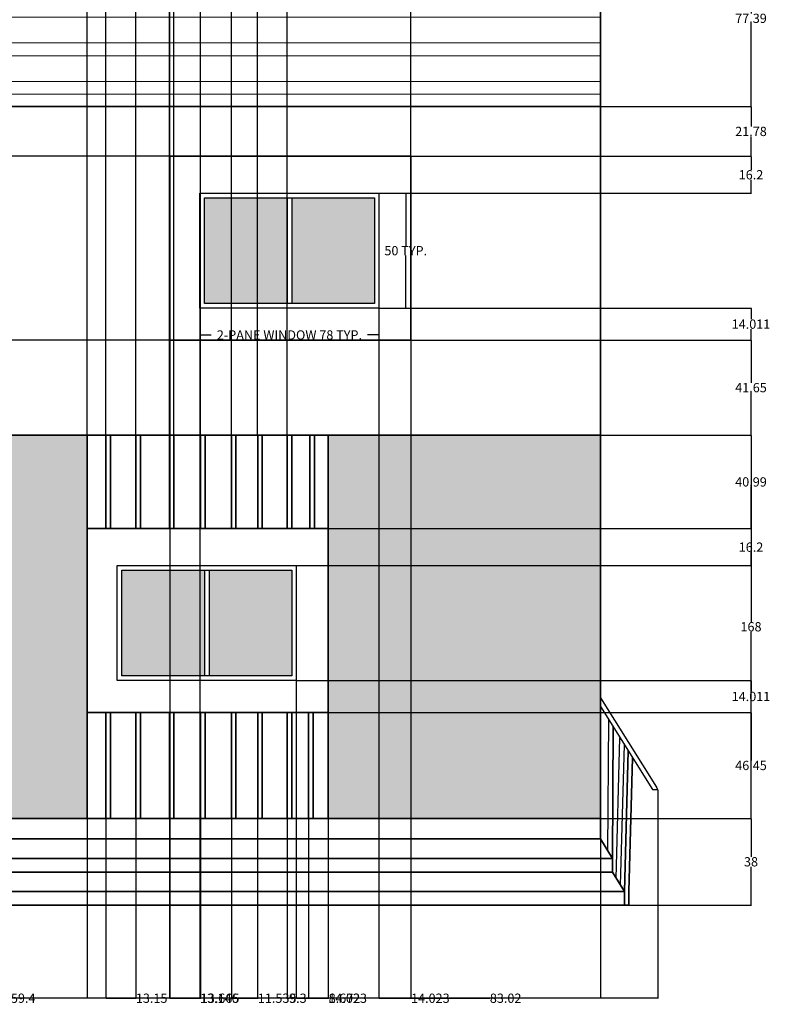
# Model space of a CAD drawing. Units: inches. Extents: x -35 to 623, y 74 to 964.
# Tile 2 of 3: x 294 to 623, y 74 to 505. Entities that reach past the tile are written whole.
import ezdxf

# ---------------------------------------------------------------- set-up
doc = ezdxf.new("R2010")
doc.units = ezdxf.units.IN
doc.header["$MEASUREMENT"] = 0
for name, color, linetype, lineweight in [('A-ANNO-DIMS', 2, 'Continuous', 18), ('A-ELEV', 7, 'Continuous', 35), ('A-ELEV-PATT', 8, 'Continuous', 13), ('A-FLOR-STRS', 7, 'Continuous', 25), ('A-GLAZ', 4, 'Continuous', 25)]:
    doc.layers.add(name, color=color, linetype=linetype, lineweight=lineweight)
doc.styles.get("Standard").update_dxf_attribs({"font": 'arial.ttf'})
doc.dimstyles.get("Standard").update_dxf_attribs({"dimtxt": 4.0625, "dimasz": 0.18, "dimexe": 0.18, "dimexo": 0.0625, "dimgap": 0.09, "dimtad": 0, "dimtih": 1, "dimtoh": 1, "dimdec": 4, "dimzin": 0, "dimdsep": 46, "dimlunit": 4, "dimtxsty": 'Standard', "dimcen": 0.09, "dimadec": 0, "dimazin": 0, "dimtfac": 1, "dimtdec": 4, "dimtofl": 0, "dimtmove": 0, "dimatfit": 3, "dimfxl": 1, "dimtolj": 1, "dimtzin": 0, "dimarcsym": 0})

# ---------------------------------------------------------------- blocks, each defined once
blk = doc.blocks.new('WIN-2PANE')
for p, q in [((38.22, 48.35), (38.22, 2)), ((40.22, 48.35), (40.22, 2))]:
    blk.add_line(p, q)
for points in [[(0, 50.35), (78.44, 50.35), (78.44, 0), (0, 0)], [(2, 48.35), (76.44, 48.35), (76.44, 2), (2, 2)]]:
    blk.add_lwpolyline(points, close=True)
blk = doc.blocks.new('STAIR-RAIL')
for p, q in [((25.22, 82.16), (0.67, 43)), ((25.22, 78.4), (2.36, 41.93)), ((21.93, 15.01), (21.56, 72.56)), ((16.35, 0), (14.7, 61.62)), ((18.27, 3.03), (16.62, 64.68)), ((0, 41.93), (0.67, 43)), ((2.36, 41.93), (0, 41.93))]:
    blk.add_line(p, q)
blk = doc.blocks.new('*D9')
at = {"layer": 'A-ANNO-DIMS', "color": 0, "lineweight": -2, "transparency": 16777216}
for p, q in [((372.93, 378.73), (372.93, 366.84)), ((451.37, 378.73), (451.37, 366.84)), ((373.11, 367.02), (377.86, 367.02)), ((451.19, 367.02), (446.44, 367.02))]:
    blk.add_line(p, q, dxfattribs=at)
at = {"layer": 'A-ANNO-DIMS', "color": 0, "transparency": 16777216}
for points in [[(373.11, 367.05), (373.11, 366.99), (372.93, 367.02)], [(451.19, 367.05), (451.19, 366.99), (451.37, 367.02)]]:
    blk.add_solid(points, dxfattribs=at)
at = {"layer": 'Defpoints', "color": 0, "transparency": 16777216}
for p in [(372.93, 378.79), (451.37, 378.79), (451.37, 367.02)]:
    blk.add_point(p, dxfattribs=at)
at = {"layer": 'A-ANNO-DIMS', "color": 0, "transparency": 16777216, "insert": (412.15, 367.02), "char_height": 4.0625, "attachment_point": 5}
blk.add_mtext('\\A1;2-PANE WINDOW 78 TYP.', dxfattribs=at)
blk = doc.blocks.new('*D10')
at = {"layer": 'A-ANNO-DIMS', "color": 0, "lineweight": -2, "transparency": 16777216}
for p, q in [((451.44, 429.14), (463.32, 429.14)), ((463.14, 428.96), (463.14, 406.13)), ((463.14, 378.97), (463.14, 401.8)), ((451.44, 378.79), (463.32, 378.79))]:
    blk.add_line(p, q, dxfattribs=at)
at = {"layer": 'A-ANNO-DIMS', "color": 0, "transparency": 16777216}
for points in [[(463.11, 428.96), (463.17, 428.96), (463.14, 429.14)], [(463.11, 378.97), (463.17, 378.97), (463.14, 378.79)]]:
    blk.add_solid(points, dxfattribs=at)
at = {"layer": 'Defpoints', "color": 0, "transparency": 16777216}
for p in [(451.37, 429.14), (463.14, 429.14), (451.37, 378.79)]:
    blk.add_point(p, dxfattribs=at)
at = {"layer": 'A-ANNO-DIMS', "color": 0, "transparency": 16777216, "insert": (463.14, 403.97), "char_height": 4.0625, "attachment_point": 5}
blk.add_mtext('\\A1;50 TYP.', dxfattribs=at)
blk = doc.blocks.new('*D13')
at = {"layer": 'A-ANNO-DIMS', "color": 0, "lineweight": -2, "transparency": 16777216}
for p, q in [((14.26, 275.06), (14.26, 76.15)), ((573.64, 167.68), (573.64, 76.15)), ((14.44, 76.33), (287.01, 76.33)), ((573.46, 76.33), (300.89, 76.33))]:
    blk.add_line(p, q, dxfattribs=at)
at = {"layer": 'A-ANNO-DIMS', "color": 0, "transparency": 16777216}
for points in [[(14.44, 76.36), (14.44, 76.3), (14.26, 76.33)], [(573.46, 76.36), (573.46, 76.3), (573.64, 76.33)]]:
    blk.add_solid(points, dxfattribs=at)
at = {"layer": 'Defpoints', "color": 0, "transparency": 16777216}
for p in [(14.26, 275.13), (573.64, 167.74), (573.64, 76.33)]:
    blk.add_point(p, dxfattribs=at)
at = {"layer": 'A-ANNO-DIMS', "color": 0, "transparency": 16777216, "insert": (293.95, 76.33), "char_height": 4.062, "attachment_point": 5}
blk.add_mtext('\\A1;559.4', dxfattribs=at)
blk = doc.blocks.new('*D23')
at = {"layer": 'A-ANNO-DIMS', "color": 0, "lineweight": -2, "transparency": 16777216}
for p, q in [((548.48, 155.13), (614.62, 155.13)), ((614.44, 154.95), (614.44, 138.29)), ((614.44, 117.31), (614.44, 133.96)), ((559.02, 117.13), (614.62, 117.13))]:
    blk.add_line(p, q, dxfattribs=at)
at = {"layer": 'A-ANNO-DIMS', "color": 0, "transparency": 16777216}
for points in [[(614.41, 154.95), (614.47, 154.95), (614.44, 155.13)], [(614.41, 117.31), (614.47, 117.31), (614.44, 117.13)]]:
    blk.add_solid(points, dxfattribs=at)
at = {"layer": 'Defpoints', "color": 0, "transparency": 16777216}
for p in [(548.42, 155.13), (614.44, 155.13), (558.95, 117.13)]:
    blk.add_point(p, dxfattribs=at)
at = {"layer": 'A-ANNO-DIMS', "color": 0, "transparency": 16777216, "insert": (614.44, 136.13), "char_height": 4.062, "attachment_point": 5}
blk.add_mtext('\\A1;38', dxfattribs=at)
blk = doc.blocks.new('*D24')
at = {"layer": 'A-ANNO-DIMS', "color": 0, "lineweight": -2, "transparency": 16777216}
for p, q in [((548.48, 323.13), (614.62, 323.13)), ((614.44, 322.95), (614.44, 241.29)), ((614.44, 155.31), (614.44, 236.96)), ((548.48, 155.13), (614.62, 155.13))]:
    blk.add_line(p, q, dxfattribs=at)
at = {"layer": 'A-ANNO-DIMS', "color": 0, "transparency": 16777216}
for points in [[(614.41, 322.95), (614.47, 322.95), (614.44, 323.13)], [(614.41, 155.31), (614.47, 155.31), (614.44, 155.13)]]:
    blk.add_solid(points, dxfattribs=at)
at = {"layer": 'Defpoints', "color": 0, "transparency": 16777216}
for p in [(548.42, 323.13), (614.44, 323.13), (548.42, 155.13)]:
    blk.add_point(p, dxfattribs=at)
at = {"layer": 'A-ANNO-DIMS', "color": 0, "transparency": 16777216, "insert": (614.44, 239.13), "char_height": 4.062, "attachment_point": 5}
blk.add_mtext('\\A1;168', dxfattribs=at)
blk = doc.blocks.new('*D25')
at = {"layer": 'A-ANNO-DIMS', "color": 0, "lineweight": -2, "transparency": 16777216}
for p, q in [((465.46, 364.78), (614.62, 364.78)), ((614.44, 364.6), (614.44, 346.12)), ((614.44, 323.31), (614.44, 341.79)), ((548.48, 323.13), (614.62, 323.13))]:
    blk.add_line(p, q, dxfattribs=at)
at = {"layer": 'A-ANNO-DIMS', "color": 0, "transparency": 16777216}
for points in [[(614.41, 364.6), (614.47, 364.6), (614.44, 364.78)], [(614.41, 323.31), (614.47, 323.31), (614.44, 323.13)]]:
    blk.add_solid(points, dxfattribs=at)
at = {"layer": 'Defpoints', "color": 0, "transparency": 16777216}
for p in [(465.4, 364.78), (614.44, 364.78), (548.42, 323.13)]:
    blk.add_point(p, dxfattribs=at)
at = {"layer": 'A-ANNO-DIMS', "color": 0, "transparency": 16777216, "insert": (614.44, 343.95), "char_height": 4.062, "attachment_point": 5}
blk.add_mtext('\\A1;41.65', dxfattribs=at)
blk = doc.blocks.new('*D26')
at = {"layer": 'A-ANNO-DIMS', "color": 0, "lineweight": -2, "transparency": 16777216}
for p, q in [((553.49, 544.52), (614.62, 544.52)), ((614.44, 544.34), (614.44, 507.99)), ((614.44, 467.31), (614.44, 503.66)), ((548.48, 467.13), (614.62, 467.13))]:
    blk.add_line(p, q, dxfattribs=at)
at = {"layer": 'A-ANNO-DIMS', "color": 0, "transparency": 16777216}
for points in [[(614.41, 544.34), (614.47, 544.34), (614.44, 544.52)], [(614.41, 467.31), (614.47, 467.31), (614.44, 467.13)]]:
    blk.add_solid(points, dxfattribs=at)
at = {"layer": 'Defpoints', "color": 0, "transparency": 16777216}
for p in [(553.43, 544.52), (614.44, 544.52), (548.42, 467.13)]:
    blk.add_point(p, dxfattribs=at)
at = {"layer": 'A-ANNO-DIMS', "color": 0, "transparency": 16777216, "insert": (614.44, 505.82), "char_height": 4.062, "attachment_point": 5}
blk.add_mtext('\\A1;77.39', dxfattribs=at)
blk = doc.blocks.new('*D47')
at = {"layer": 'A-ANNO-DIMS', "color": 0, "lineweight": -2, "transparency": 16777216}
for p, q in [((186.58, 279.26), (186.58, 76.15)), ((323.56, 155.06), (323.56, 76.15)), ((186.76, 76.33), (246.74, 76.33)), ((323.38, 76.33), (263.41, 76.33))]:
    blk.add_line(p, q, dxfattribs=at)
at = {"layer": 'A-ANNO-DIMS', "color": 0, "transparency": 16777216}
for points in [[(186.76, 76.36), (186.76, 76.3), (186.58, 76.33)], [(323.38, 76.36), (323.38, 76.3), (323.56, 76.33)]]:
    blk.add_solid(points, dxfattribs=at)
at = {"layer": 'Defpoints', "color": 0, "transparency": 16777216}
for p in [(186.58, 279.33), (323.56, 155.13), (323.56, 76.33)]:
    blk.add_point(p, dxfattribs=at)
at = {"layer": 'A-ANNO-DIMS', "color": 0, "transparency": 16777216, "insert": (255.07, 76.33), "char_height": 4.062, "attachment_point": 5}
blk.add_mtext('\\A1;136.98', dxfattribs=at)
blk = doc.blocks.new('*D48')
at = {"layer": 'A-ANNO-DIMS', "color": 0, "lineweight": -2, "transparency": 16777216}
for p, q in [((331.68, 155.06), (331.68, 76.15)), ((344.83, 155.06), (344.83, 76.15)), ((331.86, 76.33), (344.65, 76.33)), ((344.83, 76.33), (345.01, 76.33))]:
    blk.add_line(p, q, dxfattribs=at)
at = {"layer": 'A-ANNO-DIMS', "color": 0, "transparency": 16777216}
for points in [[(331.86, 76.36), (331.86, 76.3), (331.68, 76.33)], [(344.65, 76.36), (344.65, 76.3), (344.83, 76.33)]]:
    blk.add_solid(points, dxfattribs=at)
at = {"layer": 'Defpoints', "color": 0, "transparency": 16777216}
for p in [(331.68, 155.13), (344.83, 155.13), (344.83, 76.33)]:
    blk.add_point(p, dxfattribs=at)
at = {"layer": 'A-ANNO-DIMS', "color": 0, "transparency": 16777216, "insert": (351.78, 76.33), "char_height": 4.062, "attachment_point": 5}
blk.add_mtext('\\A1;13.15', dxfattribs=at)
blk = doc.blocks.new('*D49')
at = {"layer": 'A-ANNO-DIMS', "color": 0, "lineweight": -2, "transparency": 16777216}
for p, q in [((359.56, 155.06), (359.56, 76.15)), ((373.22, 155.06), (373.22, 76.15)), ((359.74, 76.33), (373.04, 76.33)), ((373.22, 76.33), (373.4, 76.33))]:
    blk.add_line(p, q, dxfattribs=at)
at = {"layer": 'A-ANNO-DIMS', "color": 0, "transparency": 16777216}
for points in [[(359.74, 76.36), (359.74, 76.3), (359.56, 76.33)], [(373.04, 76.36), (373.04, 76.3), (373.22, 76.33)]]:
    blk.add_solid(points, dxfattribs=at)
at = {"layer": 'Defpoints', "color": 0, "transparency": 16777216}
for p in [(359.56, 155.13), (373.22, 155.13), (373.22, 76.33)]:
    blk.add_point(p, dxfattribs=at)
at = {"layer": 'A-ANNO-DIMS', "color": 0, "transparency": 16777216, "insert": (381.75, 76.33), "char_height": 4.062, "attachment_point": 5}
blk.add_mtext('\\A1;13.665', dxfattribs=at)
blk = doc.blocks.new('*D50')
at = {"layer": 'A-ANNO-DIMS', "color": 0, "lineweight": -2, "transparency": 16777216}
for p, q in [((386.71, 155.06), (386.71, 76.15)), ((398.24, 155.06), (398.24, 76.15)), ((386.89, 76.33), (398.06, 76.33)), ((398.24, 76.33), (398.42, 76.33))]:
    blk.add_line(p, q, dxfattribs=at)
at = {"layer": 'A-ANNO-DIMS', "color": 0, "transparency": 16777216}
for points in [[(386.89, 76.36), (386.89, 76.3), (386.71, 76.33)], [(398.06, 76.36), (398.06, 76.3), (398.24, 76.33)]]:
    blk.add_solid(points, dxfattribs=at)
at = {"layer": 'Defpoints', "color": 0, "transparency": 16777216}
for p in [(386.71, 155.13), (398.24, 155.13), (398.24, 76.33)]:
    blk.add_point(p, dxfattribs=at)
at = {"layer": 'A-ANNO-DIMS', "color": 0, "transparency": 16777216, "insert": (406.77, 76.33), "char_height": 4.062, "attachment_point": 5}
blk.add_mtext('\\A1;11.535', dxfattribs=at)
blk = doc.blocks.new('*D51')
at = {"layer": 'A-ANNO-DIMS', "color": 0, "lineweight": -2, "transparency": 16777216}
for p, q in [((411.2, 155.06), (411.2, 76.15)), ((420.5, 155.06), (420.5, 76.15)), ((411.38, 76.33), (412.06, 76.33)), ((420.32, 76.33), (419.64, 76.33))]:
    blk.add_line(p, q, dxfattribs=at)
at = {"layer": 'A-ANNO-DIMS', "color": 0, "transparency": 16777216}
for points in [[(411.38, 76.36), (411.38, 76.3), (411.2, 76.33)], [(420.32, 76.36), (420.32, 76.3), (420.5, 76.33)]]:
    blk.add_solid(points, dxfattribs=at)
at = {"layer": 'Defpoints', "color": 0, "transparency": 16777216}
for p in [(411.2, 155.13), (420.5, 155.13), (420.5, 76.33)]:
    blk.add_point(p, dxfattribs=at)
at = {"layer": 'A-ANNO-DIMS', "color": 0, "transparency": 16777216, "insert": (415.85, 76.33), "char_height": 4.062, "attachment_point": 5}
blk.add_mtext('\\A1;9.3', dxfattribs=at)
blk = doc.blocks.new('*D52')
at = {"layer": 'A-ANNO-DIMS', "color": 0, "lineweight": -2, "transparency": 16777216}
for p, q in [((420.5, 155.06), (420.5, 76.15)), ((429.17, 155.06), (429.17, 76.15)), ((420.68, 76.33), (428.99, 76.33)), ((429.17, 76.33), (429.35, 76.33))]:
    blk.add_line(p, q, dxfattribs=at)
at = {"layer": 'A-ANNO-DIMS', "color": 0, "transparency": 16777216}
for points in [[(420.68, 76.36), (420.68, 76.3), (420.5, 76.33)], [(428.99, 76.36), (428.99, 76.3), (429.17, 76.33)]]:
    blk.add_solid(points, dxfattribs=at)
at = {"layer": 'Defpoints', "color": 0, "transparency": 16777216}
for p in [(420.5, 155.13), (429.17, 155.13), (429.17, 76.33)]:
    blk.add_point(p, dxfattribs=at)
at = {"layer": 'A-ANNO-DIMS', "color": 0, "transparency": 16777216, "insert": (436.28, 76.33), "char_height": 4.062, "attachment_point": 5}
blk.add_mtext('\\A1;8.672', dxfattribs=at)
blk = doc.blocks.new('*D53')
at = {"layer": 'A-ANNO-DIMS', "color": 0, "lineweight": -2, "transparency": 16777216}
for p, q in [((415.15, 215.52), (415.15, 76.15)), ((429.17, 201.51), (429.17, 76.15)), ((415.33, 76.33), (428.99, 76.33)), ((429.17, 76.33), (429.35, 76.33))]:
    blk.add_line(p, q, dxfattribs=at)
at = {"layer": 'A-ANNO-DIMS', "color": 0, "transparency": 16777216}
for points in [[(415.33, 76.36), (415.33, 76.3), (415.15, 76.33)], [(428.99, 76.36), (428.99, 76.3), (429.17, 76.33)]]:
    blk.add_solid(points, dxfattribs=at)
at = {"layer": 'Defpoints', "color": 0, "transparency": 16777216}
for p in [(415.15, 215.58), (429.17, 201.57), (429.17, 76.33)]:
    blk.add_point(p, dxfattribs=at)
at = {"layer": 'A-ANNO-DIMS', "color": 0, "transparency": 16777216, "insert": (437.68, 76.33), "char_height": 4.062, "attachment_point": 5}
blk.add_mtext('\\A1;14.023', dxfattribs=at)
blk = doc.blocks.new('*D58')
at = {"layer": 'A-ANNO-DIMS', "color": 0, "lineweight": -2, "transparency": 16777216}
for p, q in [((323.56, 323.19), (323.56, 961.9)), ((323.74, 961.72), (331.5, 961.72)), ((331.68, 323.19), (331.68, 961.9)), ((331.68, 961.72), (331.86, 961.72))]:
    blk.add_line(p, q, dxfattribs=at)
at = {"layer": 'A-ANNO-DIMS', "color": 0, "transparency": 16777216}
for points in [[(323.74, 961.75), (323.74, 961.69), (323.56, 961.72)], [(331.5, 961.75), (331.5, 961.69), (331.68, 961.72)]]:
    blk.add_solid(points, dxfattribs=at)
at = {"layer": 'Defpoints', "color": 0, "transparency": 16777216}
for p in [(331.68, 961.72), (323.56, 323.13), (331.68, 323.13)]:
    blk.add_point(p, dxfattribs=at)
at = {"layer": 'A-ANNO-DIMS', "color": 0, "transparency": 16777216, "insert": (338.8, 961.72), "char_height": 4.062, "attachment_point": 5}
blk.add_mtext('\\A1;8.114', dxfattribs=at)
blk = doc.blocks.new('*D59')
at = {"layer": 'A-ANNO-DIMS', "color": 0, "lineweight": -2, "transparency": 16777216}
for p, q in [((344.83, 323.19), (344.83, 961.9)), ((345.01, 961.72), (345.44, 961.72)), ((359.38, 961.72), (358.95, 961.72)), ((359.56, 323.19), (359.56, 961.9))]:
    blk.add_line(p, q, dxfattribs=at)
at = {"layer": 'A-ANNO-DIMS', "color": 0, "transparency": 16777216}
for points in [[(345.01, 961.75), (345.01, 961.69), (344.83, 961.72)], [(359.38, 961.75), (359.38, 961.69), (359.56, 961.72)]]:
    blk.add_solid(points, dxfattribs=at)
at = {"layer": 'Defpoints', "color": 0, "transparency": 16777216}
for p in [(359.56, 961.72), (344.83, 323.13), (359.56, 323.13)]:
    blk.add_point(p, dxfattribs=at)
at = {"layer": 'A-ANNO-DIMS', "color": 0, "transparency": 16777216, "insert": (352.19, 961.72), "char_height": 4.062, "attachment_point": 5}
blk.add_mtext('\\A1;14.73', dxfattribs=at)
blk = doc.blocks.new('*D60')
at = {"layer": 'A-ANNO-DIMS', "color": 0, "lineweight": -2, "transparency": 16777216}
for p, q in [((359.56, 323.19), (359.56, 961.9)), ((359.74, 961.72), (361.38, 961.72)), ((361.56, 323.19), (361.56, 961.9)), ((361.56, 961.72), (361.74, 961.72))]:
    blk.add_line(p, q, dxfattribs=at)
at = {"layer": 'A-ANNO-DIMS', "color": 0, "transparency": 16777216}
for points in [[(359.74, 961.75), (359.74, 961.69), (359.56, 961.72)], [(361.38, 961.75), (361.38, 961.69), (361.56, 961.72)]]:
    blk.add_solid(points, dxfattribs=at)
at = {"layer": 'Defpoints', "color": 0, "transparency": 16777216}
for p in [(361.56, 961.72), (359.56, 323.13), (361.56, 323.13)]:
    blk.add_point(p, dxfattribs=at)
at = {"layer": 'A-ANNO-DIMS', "color": 0, "transparency": 16777216, "insert": (363.17, 961.72), "char_height": 4.062, "attachment_point": 5}
blk.add_mtext('\\A1;2', dxfattribs=at)
blk = doc.blocks.new('*D61')
at = {"layer": 'A-ANNO-DIMS', "color": 0, "lineweight": -2, "transparency": 16777216}
for p, q in [((373.22, 323.19), (373.22, 961.9)), ((373.4, 961.72), (386.53, 961.72)), ((386.71, 323.19), (386.71, 961.9)), ((386.71, 961.72), (386.89, 961.72))]:
    blk.add_line(p, q, dxfattribs=at)
at = {"layer": 'A-ANNO-DIMS', "color": 0, "transparency": 16777216}
for points in [[(373.4, 961.75), (373.4, 961.69), (373.22, 961.72)], [(386.53, 961.75), (386.53, 961.69), (386.71, 961.72)]]:
    blk.add_solid(points, dxfattribs=at)
at = {"layer": 'Defpoints', "color": 0, "transparency": 16777216}
for p in [(386.71, 961.72), (373.22, 323.13), (386.71, 323.13)]:
    blk.add_point(p, dxfattribs=at)
at = {"layer": 'A-ANNO-DIMS', "color": 0, "transparency": 16777216, "insert": (395.22, 961.72), "char_height": 4.062, "attachment_point": 5}
blk.add_mtext('\\A1;13.487', dxfattribs=at)
blk = doc.blocks.new('*D62')
at = {"layer": 'A-ANNO-DIMS', "color": 0, "lineweight": -2, "transparency": 16777216}
for p, q in [((398.24, 323.19), (398.24, 961.9)), ((398.42, 961.72), (411.02, 961.72)), ((411.2, 323.19), (411.2, 961.9)), ((411.2, 961.72), (411.38, 961.72))]:
    blk.add_line(p, q, dxfattribs=at)
at = {"layer": 'A-ANNO-DIMS', "color": 0, "transparency": 16777216}
for points in [[(398.42, 961.75), (398.42, 961.69), (398.24, 961.72)], [(411.02, 961.75), (411.02, 961.69), (411.2, 961.72)]]:
    blk.add_solid(points, dxfattribs=at)
at = {"layer": 'Defpoints', "color": 0, "transparency": 16777216}
for p in [(411.2, 961.72), (398.24, 323.13), (411.2, 323.13)]:
    blk.add_point(p, dxfattribs=at)
at = {"layer": 'A-ANNO-DIMS', "color": 0, "transparency": 16777216, "insert": (419.73, 961.72), "char_height": 4.062, "attachment_point": 5}
blk.add_mtext('\\A1;12.955', dxfattribs=at)
blk = doc.blocks.new('*D63')
at = {"layer": 'A-ANNO-DIMS', "color": 0, "lineweight": -2, "transparency": 16777216}
for p, q in [((429.23, 201.57), (614.62, 201.57)), ((614.44, 201.39), (614.44, 180.51)), ((614.44, 155.31), (614.44, 176.18)), ((429.23, 155.13), (614.62, 155.13))]:
    blk.add_line(p, q, dxfattribs=at)
at = {"layer": 'A-ANNO-DIMS', "color": 0, "transparency": 16777216}
for points in [[(614.41, 201.39), (614.47, 201.39), (614.44, 201.57)], [(614.41, 155.31), (614.47, 155.31), (614.44, 155.13)]]:
    blk.add_solid(points, dxfattribs=at)
at = {"layer": 'Defpoints', "color": 0, "transparency": 16777216}
for p in [(429.17, 201.57), (614.44, 201.57), (429.17, 155.13)]:
    blk.add_point(p, dxfattribs=at)
at = {"layer": 'A-ANNO-DIMS', "color": 0, "transparency": 16777216, "insert": (614.44, 178.35), "char_height": 4.062, "attachment_point": 5}
blk.add_mtext('\\A1;46.45', dxfattribs=at)
blk = doc.blocks.new('*D64')
at = {"layer": 'A-ANNO-DIMS', "color": 0, "lineweight": -2, "transparency": 16777216}
for p, q in [((415.21, 215.58), (614.62, 215.58)), ((614.44, 215.4), (614.44, 210.74)), ((614.44, 201.75), (614.44, 206.41)), ((429.23, 201.57), (614.62, 201.57))]:
    blk.add_line(p, q, dxfattribs=at)
at = {"layer": 'A-ANNO-DIMS', "color": 0, "transparency": 16777216}
for points in [[(614.41, 215.4), (614.47, 215.4), (614.44, 215.58)], [(614.41, 201.75), (614.47, 201.75), (614.44, 201.57)]]:
    blk.add_solid(points, dxfattribs=at)
at = {"layer": 'Defpoints', "color": 0, "transparency": 16777216}
for p in [(415.15, 215.58), (614.44, 215.58), (429.17, 201.57)]:
    blk.add_point(p, dxfattribs=at)
at = {"layer": 'A-ANNO-DIMS', "color": 0, "transparency": 16777216, "insert": (614.44, 208.58), "char_height": 4.062, "attachment_point": 5}
blk.add_mtext('\\A1;14.011', dxfattribs=at)
blk = doc.blocks.new('*D65')
at = {"layer": 'A-ANNO-DIMS', "color": 0, "lineweight": -2, "transparency": 16777216}
for p, q in [((429.23, 282.14), (614.62, 282.14)), ((614.44, 281.96), (614.44, 276.2)), ((614.44, 266.12), (614.44, 271.87)), ((415.21, 265.94), (614.62, 265.94))]:
    blk.add_line(p, q, dxfattribs=at)
at = {"layer": 'A-ANNO-DIMS', "color": 0, "transparency": 16777216}
for points in [[(614.41, 281.96), (614.47, 281.96), (614.44, 282.14)], [(614.41, 266.12), (614.47, 266.12), (614.44, 265.94)]]:
    blk.add_solid(points, dxfattribs=at)
at = {"layer": 'Defpoints', "color": 0, "transparency": 16777216}
for p in [(429.17, 282.14), (614.44, 282.14), (415.15, 265.94)]:
    blk.add_point(p, dxfattribs=at)
at = {"layer": 'A-ANNO-DIMS', "color": 0, "transparency": 16777216, "insert": (614.44, 274.04), "char_height": 4.062, "attachment_point": 5}
blk.add_mtext('\\A1;16.2', dxfattribs=at)
blk = doc.blocks.new('*D66')
at = {"layer": 'A-ANNO-DIMS', "color": 0, "lineweight": -2, "transparency": 16777216}
for p, q in [((429.23, 323.13), (614.62, 323.13)), ((614.44, 322.95), (614.44, 304.8)), ((614.44, 282.32), (614.44, 300.47)), ((429.23, 282.14), (614.62, 282.14))]:
    blk.add_line(p, q, dxfattribs=at)
at = {"layer": 'A-ANNO-DIMS', "color": 0, "transparency": 16777216}
for points in [[(614.41, 322.95), (614.47, 322.95), (614.44, 323.13)], [(614.41, 282.32), (614.47, 282.32), (614.44, 282.14)]]:
    blk.add_solid(points, dxfattribs=at)
at = {"layer": 'Defpoints', "color": 0, "transparency": 16777216}
for p in [(429.17, 323.13), (614.44, 323.13), (429.17, 282.14)]:
    blk.add_point(p, dxfattribs=at)
at = {"layer": 'A-ANNO-DIMS', "color": 0, "transparency": 16777216, "insert": (614.44, 302.63), "char_height": 4.062, "attachment_point": 5}
blk.add_mtext('\\A1;40.99', dxfattribs=at)
blk = doc.blocks.new('*D67')
at = {"layer": 'A-ANNO-DIMS', "color": 0, "lineweight": -2, "transparency": 16777216}
for p, q in [((372.93, 378.73), (372.93, 76.15)), ((359.79, 364.72), (359.79, 76.15)), ((359.97, 76.33), (372.75, 76.33)), ((372.93, 76.33), (373.11, 76.33))]:
    blk.add_line(p, q, dxfattribs=at)
at = {"layer": 'A-ANNO-DIMS', "color": 0, "transparency": 16777216}
for points in [[(359.97, 76.36), (359.97, 76.3), (359.79, 76.33)], [(372.75, 76.36), (372.75, 76.3), (372.93, 76.33)]]:
    blk.add_solid(points, dxfattribs=at)
at = {"layer": 'Defpoints', "color": 0, "transparency": 16777216}
for p in [(372.93, 378.79), (359.79, 364.78), (372.93, 76.33)]:
    blk.add_point(p, dxfattribs=at)
at = {"layer": 'A-ANNO-DIMS', "color": 0, "transparency": 16777216, "insert": (381.44, 76.33), "char_height": 4.062, "attachment_point": 5}
blk.add_mtext('\\A1;13.146', dxfattribs=at)
blk = doc.blocks.new('*D68')
at = {"layer": 'A-ANNO-DIMS', "color": 0, "lineweight": -2, "transparency": 16777216}
for p, q in [((451.37, 378.73), (451.37, 76.15)), ((465.4, 364.72), (465.4, 76.15)), ((451.55, 76.33), (465.22, 76.33)), ((465.4, 76.33), (465.58, 76.33))]:
    blk.add_line(p, q, dxfattribs=at)
at = {"layer": 'A-ANNO-DIMS', "color": 0, "transparency": 16777216}
for points in [[(451.55, 76.36), (451.55, 76.3), (451.37, 76.33)], [(465.22, 76.36), (465.22, 76.3), (465.4, 76.33)]]:
    blk.add_solid(points, dxfattribs=at)
at = {"layer": 'Defpoints', "color": 0, "transparency": 16777216}
for p in [(451.37, 378.79), (465.4, 364.78), (465.4, 76.33)]:
    blk.add_point(p, dxfattribs=at)
at = {"layer": 'A-ANNO-DIMS', "color": 0, "transparency": 16777216, "insert": (473.91, 76.33), "char_height": 4.062, "attachment_point": 5}
blk.add_mtext('\\A1;14.023', dxfattribs=at)
blk = doc.blocks.new('*D69')
at = {"layer": 'A-ANNO-DIMS', "color": 0, "lineweight": -2, "transparency": 16777216}
for p, q in [((548.42, 467.06), (548.42, 76.15)), ((465.4, 364.72), (465.4, 76.15)), ((465.58, 76.33), (499.98, 76.33)), ((548.24, 76.33), (513.83, 76.33))]:
    blk.add_line(p, q, dxfattribs=at)
at = {"layer": 'A-ANNO-DIMS', "color": 0, "transparency": 16777216}
for points in [[(465.58, 76.36), (465.58, 76.3), (465.4, 76.33)], [(548.24, 76.36), (548.24, 76.3), (548.42, 76.33)]]:
    blk.add_solid(points, dxfattribs=at)
at = {"layer": 'Defpoints', "color": 0, "transparency": 16777216}
for p in [(548.42, 467.13), (465.4, 364.78), (548.42, 76.33)]:
    blk.add_point(p, dxfattribs=at)
at = {"layer": 'A-ANNO-DIMS', "color": 0, "transparency": 16777216, "insert": (506.91, 76.33), "char_height": 4.062, "attachment_point": 5}
blk.add_mtext('\\A1;83.02', dxfattribs=at)
blk = doc.blocks.new('*D70')
at = {"layer": 'A-ANNO-DIMS', "color": 0, "lineweight": -2, "transparency": 16777216}
for p, q in [((359.79, 445.41), (359.79, 961.9)), ((359.97, 961.72), (405.84, 961.72)), ((465.22, 961.72), (419.34, 961.72)), ((465.4, 445.41), (465.4, 961.9))]:
    blk.add_line(p, q, dxfattribs=at)
at = {"layer": 'A-ANNO-DIMS', "color": 0, "transparency": 16777216}
for points in [[(359.97, 961.75), (359.97, 961.69), (359.79, 961.72)], [(465.22, 961.75), (465.22, 961.69), (465.4, 961.72)]]:
    blk.add_solid(points, dxfattribs=at)
at = {"layer": 'Defpoints', "color": 0, "transparency": 16777216}
for p in [(465.4, 961.72), (359.79, 445.34), (465.4, 445.34)]:
    blk.add_point(p, dxfattribs=at)
at = {"layer": 'A-ANNO-DIMS', "color": 0, "transparency": 16777216, "insert": (412.59, 961.72), "char_height": 4.062, "attachment_point": 5}
blk.add_mtext('\\A1;105.6', dxfattribs=at)
blk = doc.blocks.new('*D71')
at = {"layer": 'A-ANNO-DIMS', "color": 0, "lineweight": -2, "transparency": 16777216}
for p, q in [((451.44, 378.79), (614.62, 378.79)), ((614.44, 378.61), (614.44, 373.95)), ((614.44, 364.96), (614.44, 369.62)), ((465.46, 364.78), (614.62, 364.78))]:
    blk.add_line(p, q, dxfattribs=at)
at = {"layer": 'A-ANNO-DIMS', "color": 0, "transparency": 16777216}
for points in [[(614.41, 378.61), (614.47, 378.61), (614.44, 378.79)], [(614.41, 364.96), (614.47, 364.96), (614.44, 364.78)]]:
    blk.add_solid(points, dxfattribs=at)
at = {"layer": 'Defpoints', "color": 0, "transparency": 16777216}
for p in [(451.37, 378.79), (614.44, 378.79), (465.4, 364.78)]:
    blk.add_point(p, dxfattribs=at)
at = {"layer": 'A-ANNO-DIMS', "color": 0, "transparency": 16777216, "insert": (614.44, 371.78), "char_height": 4.062, "attachment_point": 5}
blk.add_mtext('\\A1;14.011', dxfattribs=at)
blk = doc.blocks.new('*D72')
at = {"layer": 'A-ANNO-DIMS', "color": 0, "lineweight": -2, "transparency": 16777216}
for p, q in [((465.46, 445.34), (614.62, 445.34)), ((614.44, 445.16), (614.44, 439.41)), ((614.44, 429.32), (614.44, 435.08)), ((451.44, 429.14), (614.62, 429.14))]:
    blk.add_line(p, q, dxfattribs=at)
at = {"layer": 'A-ANNO-DIMS', "color": 0, "transparency": 16777216}
for points in [[(614.41, 445.16), (614.47, 445.16), (614.44, 445.34)], [(614.41, 429.32), (614.47, 429.32), (614.44, 429.14)]]:
    blk.add_solid(points, dxfattribs=at)
at = {"layer": 'Defpoints', "color": 0, "transparency": 16777216}
for p in [(465.4, 445.34), (614.44, 445.34), (451.37, 429.14)]:
    blk.add_point(p, dxfattribs=at)
at = {"layer": 'A-ANNO-DIMS', "color": 0, "transparency": 16777216, "insert": (614.44, 437.24), "char_height": 4.062, "attachment_point": 5}
blk.add_mtext('\\A1;16.2', dxfattribs=at)
blk = doc.blocks.new('*D73')
at = {"layer": 'A-ANNO-DIMS', "color": 0, "lineweight": -2, "transparency": 16777216}
for p, q in [((548.48, 467.13), (614.62, 467.13)), ((614.44, 466.95), (614.44, 458.4)), ((614.44, 445.52), (614.44, 454.07)), ((465.46, 445.34), (614.62, 445.34))]:
    blk.add_line(p, q, dxfattribs=at)
at = {"layer": 'A-ANNO-DIMS', "color": 0, "transparency": 16777216}
for points in [[(614.41, 466.95), (614.47, 466.95), (614.44, 467.13)], [(614.41, 445.52), (614.47, 445.52), (614.44, 445.34)]]:
    blk.add_solid(points, dxfattribs=at)
at = {"layer": 'Defpoints', "color": 0, "transparency": 16777216}
for p in [(548.42, 467.13), (614.44, 467.13), (465.4, 445.34)]:
    blk.add_point(p, dxfattribs=at)
at = {"layer": 'A-ANNO-DIMS', "color": 0, "transparency": 16777216, "insert": (614.44, 456.24), "char_height": 4.062, "attachment_point": 5}
blk.add_mtext('\\A1;21.78', dxfattribs=at)
blk = doc.blocks.new('*D74')
at = {"layer": 'A-ANNO-DIMS', "color": 0, "lineweight": -2, "transparency": 16777216}
for p, q in [((359.73, 445.34), (-26.72, 445.34)), ((-26.54, 445.16), (-26.54, 407.23)), ((-26.54, 364.96), (-26.54, 402.9)), ((359.73, 364.78), (-26.72, 364.78))]:
    blk.add_line(p, q, dxfattribs=at)
at = {"layer": 'A-ANNO-DIMS', "color": 0, "transparency": 16777216}
for points in [[(-26.57, 445.16), (-26.51, 445.16), (-26.54, 445.34)], [(-26.57, 364.96), (-26.51, 364.96), (-26.54, 364.78)]]:
    blk.add_solid(points, dxfattribs=at)
at = {"layer": 'Defpoints', "color": 0, "transparency": 16777216}
for p in [(-26.54, 445.34), (359.79, 445.34), (359.79, 364.78)]:
    blk.add_point(p, dxfattribs=at)
at = {"layer": 'A-ANNO-DIMS', "color": 0, "transparency": 16777216, "insert": (-26.54, 405.06), "char_height": 4.062, "attachment_point": 5}
blk.add_mtext('\\A1;80.57', dxfattribs=at)

msp = doc.modelspace()

# ---------------------------------------------------------------- hatches: boundary and pattern name
at = {"layer": 'A-ELEV-PATT'}
h = msp.add_hatch(color=256, dxfattribs=at)
h.dxf.hatch_style = 1
h.set_gradient(color2=(99, 100, 102))
h.paths.add_polyline_path([(471.0064, 631.4927), (434.7868, 631.4927), (434.7868, 579.8536), (471.0064, 579.8536)])
h.paths.add_polyline_path([(509.226, 631.4927), (473.0064, 631.4927), (473.0064, 579.8536), (509.226, 579.8536)])
h.paths.add_polyline_path([(449.3739, 427.1438), (413.1543, 427.1438), (413.1543, 380.7902), (449.3739, 380.7902)])
h.paths.add_polyline_path([(411.1543, 427.1438), (374.9347, 427.1438), (374.9347, 380.7902), (411.1543, 380.7902)])
h.paths.add_polyline_path([(374.9294, 263.937), (338.7098, 263.937), (338.7098, 217.5834), (374.9294, 217.5834)])
h.paths.add_polyline_path([(413.1491, 263.937), (376.9294, 263.937), (376.9294, 217.5834), (413.1491, 217.5834)])
h.paths.add_polyline_path([(230.0086, 434.3669), (185.9817, 434.3669), (185.9817, 426.9441), (230.0086, 426.9441)])
h.paths.add_polyline_path([(230.0086, 443.5602), (185.9817, 443.5602), (185.9817, 434.3669), (230.0086, 434.3669)])
h.paths.add_polyline_path([(230.0086, 426.9441), (185.9817, 426.9441), (185.9817, 422.542), (230.0086, 422.542)])
h.paths.add_polyline_path([(230.0086, 648.8148), (185.9817, 648.8148), (185.9817, 642.5298), (230.0086, 642.5298)])
h.paths.add_polyline_path([(230.0086, 642.5298), (185.9817, 642.5298), (185.9817, 633.9381), (230.0086, 633.9381)])
h.paths.add_polyline_path([(230.0086, 633.9381), (185.9817, 633.9381), (185.9817, 627.7966), (230.0086, 627.7966)])
h.paths.add_polyline_path([(230.0086, 863.7512), (185.9817, 863.7512), (185.9817, 856.0022), (230.0086, 856.0022)])
h.paths.add_polyline_path([(230.0086, 856.0022), (185.9817, 856.0022), (185.9817, 849.1652), (230.0086, 849.1652)])
h.paths.add_polyline_path([(230.0086, 849.1652), (185.9817, 849.1652), (185.9817, 842.733), (230.0086, 842.733)])
h = msp.add_hatch(dxfattribs=at)
h.set_pattern_fill('ANSI32', color=256, scale=45, angle=135)
h.paths.add_polyline_path([(548.4175, 755.1261), (152.2908, 755.1261), (152.2908, 611.1261), (152.2908, 467.1261), (548.4175, 467.1261), (548.4175, 544.5164), (425.7698, 544.5164), (425.7698, 649.844), (548.4175, 649.844)])
h.paths.add_polyline_path([(232.0086, 650.8148), (232.0086, 625.7966), (183.9817, 625.7966), (183.9817, 650.8148)], flags=16)
h.paths.add_polyline_path([(230.0086, 648.8148), (230.0086, 627.7966), (185.9817, 627.7966), (185.9817, 648.8148)], flags=0)
h = msp.add_hatch(color=256, dxfattribs=at)
h.dxf.hatch_style = 1
h.set_gradient(color1=(199, 200, 202), color2=(99, 100, 102))
h.paths.add_polyline_path([(323.5636, 282.1377), (323.5636, 323.1261), (186.5792, 323.1261), (186.5792, 279.3267), (177.6113, 275.1261), (177.6113, 155.1261), (323.5636, 155.1261), (323.5636, 201.572)])
h.paths.add_polyline_path([(548.4175, 323.1261), (429.1717, 323.1261), (429.1717, 282.1377), (429.1717, 201.572), (429.1717, 155.1261), (548.4175, 155.1261)])
h.paths.add_polyline_path([(115.3998, 275.1261), (40.4435, 275.1261), (40.4435, 155.1261), (115.3998, 155.1261), (115.3998, 159.0807)])
h.paths.add_polyline_path([(126.5574, 273.1261), (117.3998, 273.1261), (117.3998, 161.0807), (171.3498, 161.0807), (171.3498, 210.0445), (165.6209, 210.0445), (165.6209, 208.3223), (164.9007, 208.3223), (164.9007, 210.0445), (163.8747, 210.0445), (163.8747, 172.7632), (161.5924, 172.7632), (161.5924, 210.0445), (158.6465, 210.0445), (158.6465, 211.5523), (161.5924, 211.5523), (161.5924, 273.1261), (156.6973, 273.1261), (156.6973, 172.7632), (154.4151, 172.7632), (154.4151, 273.1261), (150.4171, 273.1261), (150.4171, 172.7632), (148.1349, 172.7632), (148.1349, 273.1261), (142.7413, 273.1261), (142.7413, 172.7632), (140.4591, 172.7632), (140.4591, 273.1261), (136.1621, 273.1261), (136.1621, 172.7632), (133.8798, 172.7632), (133.8798, 273.1261), (128.8396, 273.1261), (128.8396, 172.7632), (126.5574, 172.7632)])
h.paths.add_polyline_path([(171.3498, 273.1261), (163.8747, 273.1261), (163.8747, 211.5523), (164.9007, 211.5523), (164.9007, 212.2403), (165.6209, 212.2403), (165.6209, 211.5523), (171.3498, 211.5523)], flags=17)
h.paths.add_polyline_path([(186.5792, 323.1261), (177.6113, 323.1261), (177.6113, 275.1261), (186.5792, 279.3267)], flags=17)

# ---------------------------------------------------------------- linework, layer by layer
at = {"layer": 'A-ELEV'}
for p, q in [((548.4175, 467.1261), (548.4175, 544.5164)), ((152.2908, 467.1261), (548.4175, 467.1261)), ((548.4175, 467.1261), (548.4175, 323.1261)), ((548.4175, 323.1261), (177.6113, 323.1261)), ((323.5636, 282.1377), (323.5636, 323.1261)), ((331.6772, 323.1261), (331.6772, 282.1377)), ((333.6772, 323.1261), (333.6772, 282.1377)), ((344.8278, 323.1261), (344.8278, 282.1377)), ((346.8278, 323.1261), (346.8278, 282.1377)), ((359.5574, 323.1261), (359.5574, 282.1377)), ((361.5574, 323.1261), (361.5574, 282.1377)), ((373.2221, 323.1261), (373.2221, 282.1377)), ((375.2221, 323.1261), (375.2221, 282.1377)), ((386.7094, 323.1261), (386.7094, 282.1377)), ((388.7094, 323.1261), (388.7094, 282.1377)), ((398.2446, 323.1261), (398.2446, 282.1377)), ((400.2446, 323.1261), (400.2446, 282.1377)), ((411.1995, 323.1261), (411.1995, 282.1377)), ((413.1995, 323.1261), (413.1995, 282.1377)), ((421.122, 323.1261), (421.122, 282.1377)), ((423.122, 323.1261), (423.122, 282.1377)), ((429.1717, 282.1377), (429.1717, 323.1261)), ((548.4175, 155.1261), (548.4175, 323.1261)), ((323.5636, 201.572), (323.5636, 155.1261)), ((331.6772, 201.572), (331.6772, 160.5836)), ((331.6772, 155.1261), (331.6772, 199.3827)), ((333.6772, 201.572), (333.6772, 160.5836)), ((333.6772, 155.1261), (333.6772, 199.3827)), ((344.8278, 155.1261), (344.8278, 201.572)), ((346.8278, 155.1261), (346.8278, 201.572)), ((359.5574, 155.1261), (359.5574, 201.572)), ((361.5574, 155.1261), (361.5574, 201.572)), ((373.2221, 155.1261), (373.2221, 201.572)), ((375.2221, 155.1261), (375.2221, 201.572)), ((386.7094, 155.1261), (386.7094, 201.572)), ((388.7094, 155.1261), (388.7094, 201.572)), ((398.2446, 155.1261), (398.2446, 201.572)), ((400.2446, 155.1261), (400.2446, 201.572)), ((411.1995, 155.1261), (411.1995, 201.572)), ((413.1995, 155.1261), (413.1995, 201.572)), ((420.4995, 155.1261), (420.4995, 201.572)), ((422.4995, 155.1261), (422.4995, 201.572)), ((429.1717, 201.572), (429.1717, 155.1261)), ((553.6861, 137.6266), (554.0584, 195.2104)), ((558.9547, 123.127), (560.5992, 184.7782)), ((560.954, 123.0737), (562.5183, 181.7174)), ((40.4435, 155.1261), (548.4175, 155.1261)), ((548.4175, 155.1261), (548.4175, 146.1261)), ((40.4435, 146.1261), (548.4175, 146.1261)), ((548.4175, 146.1261), (553.6861, 137.6266)), ((35.175, 137.6266), (553.6861, 137.6266)), ((553.6861, 131.6266), (553.6861, 137.6266)), ((35.175, 131.6266), (553.6861, 131.6266)), ((553.6861, 131.6266), (558.9547, 123.127)), ((29.9064, 123.127), (558.9547, 123.127)), ((558.9547, 123.127), (558.9547, 117.127)), ((560.954, 123.0737), (560.954, 117.127)), ((558.9547, 117.127), (29.9064, 117.127)), ((560.954, 117.127), (558.9547, 117.127))]:
    msp.add_line(p, q, dxfattribs=at)
for points in [[(359.7884, 445.3445), (465.3966, 445.3445), (465.3966, 364.7788), (359.7884, 364.7788)], [(323.5636, 282.1377), (429.1717, 282.1377), (429.1717, 201.572), (323.5636, 201.572)]]:
    msp.add_lwpolyline(points, close=True, dxfattribs=at)

# ---------------------------------------------------------------- block references
at = {"layer": 'A-FLOR-STRS', "extrusion": (0, 0, -1), "zscale": -1}
msp.add_blockref('STAIR-RAIL', (-573.64, 125.81), dxfattribs=at)
at = {"layer": 'A-GLAZ'}
for p in [(372.9348, 378.7898), (336.71, 215.583)]:
    msp.add_blockref('WIN-2PANE', p, dxfattribs=at)

# ---------------------------------------------------------------- dimensions: what is measured, and where the dimension line sits
at = {"layer": 'A-ANNO-DIMS'}
for base, p1, p2, override, picture, middle in [((331.6772, 961.7156), (323.5636, 323.1261), (331.6772, 323.1261), {"dimdec": 3, "dimlfac": 1, "dimrnd": 0, "dimzin": 0, "dimdsep": 46, "dimlunit": 2}, '*D58', (338.7961, 961.7156)), ((359.5574, 961.7156), (344.8278, 323.1261), (359.5574, 323.1261), {"dimdec": 2, "dimlfac": 1, "dimrnd": 0, "dimzin": 0, "dimdsep": 46, "dimlunit": 2}, '*D59', (352.1926, 961.7156)), ((361.5574, 961.7156), (359.5574, 323.1261), (361.5574, 323.1261), {"dimdec": 0, "dimlfac": 1, "dimrnd": 0, "dimzin": 0, "dimdsep": 46, "dimlunit": 2}, '*D60', (363.1727, 961.7156)), ((465.3966, 961.7156), (359.7884, 445.3445), (465.3966, 445.3445), {"dimdec": 1, "dimlfac": 1, "dimrnd": 0, "dimzin": 0, "dimdsep": 46, "dimlunit": 2}, '*D70', (412.5925, 961.7156)), ((386.7094, 961.7156), (373.2221, 323.1261), (386.7094, 323.1261), {"dimdec": 3, "dimlfac": 1, "dimrnd": 0, "dimzin": 0, "dimdsep": 46, "dimlunit": 2}, '*D61', (395.2208, 961.7156)), ((411.1995, 961.7156), (398.2446, 323.1261), (411.1995, 323.1261), {"dimdec": 3, "dimlfac": 1, "dimrnd": 0, "dimzin": 0, "dimdsep": 46, "dimlunit": 2}, '*D62', (419.7261, 961.7156)), ((548.4175, 76.327), (465.3966, 364.7788), (548.4175, 467.1261), {"dimdec": 2, "dimlfac": 1, "dimrnd": 0, "dimzin": 0, "dimdsep": 46, "dimlunit": 2}, '*D69', (506.907, 76.327)), ((372.9347, 76.327), (359.7884, 364.7788), (372.9347, 378.7902), {"dimdec": 3, "dimlfac": 1, "dimrnd": 0, "dimzin": 0, "dimdsep": 46, "dimlunit": 2}, '*D67', (381.4447, 76.327)), ((465.3966, 76.327), (451.3739, 378.7902), (465.3966, 364.7788), {"dimdec": 3, "dimlfac": 1, "dimrnd": 0, "dimzin": 0, "dimdsep": 46, "dimlunit": 2}, '*D68', (473.908, 76.327)), ((323.5636, 76.327), (186.5792, 279.3267), (323.5636, 155.1261), {"dimdec": 2, "dimlfac": 1, "dimrnd": 0, "dimzin": 0, "dimdsep": 46, "dimlunit": 2}, '*D47', (255.0714, 76.327)), ((573.6397, 76.327), (14.262, 275.1261), (573.6397, 167.7443), {"dimdec": 1, "dimlfac": 1, "dimrnd": 0, "dimzin": 0, "dimdsep": 46, "dimlunit": 2}, '*D13', (293.9509, 76.327)), ((429.1717, 76.327), (415.1491, 215.5834), (429.1717, 201.572), {"dimdec": 3, "dimlfac": 1, "dimrnd": 0, "dimzin": 0, "dimdsep": 46, "dimlunit": 2}, '*D53', (437.6831, 76.327)), ((344.8278, 76.327), (331.6772, 155.1261), (344.8278, 155.1261), {"dimdec": 2, "dimlfac": 1, "dimrnd": 0, "dimzin": 0, "dimdsep": 46, "dimlunit": 2}, '*D48', (351.7763, 76.327)), ((373.2221, 76.327), (359.5574, 155.1261), (373.2221, 155.1261), {"dimdec": 3, "dimlfac": 1, "dimrnd": 0, "dimzin": 0, "dimdsep": 46, "dimlunit": 2}, '*D49', (381.7487, 76.327)), ((398.2446, 76.327), (386.7094, 155.1261), (398.2446, 155.1261), {"dimdec": 3, "dimlfac": 1, "dimrnd": 0, "dimzin": 0, "dimdsep": 46, "dimlunit": 2}, '*D50', (406.7712, 76.327)), ((420.4995, 76.327), (411.1995, 155.1261), (420.4995, 155.1261), {"dimdec": 1, "dimlfac": 1, "dimrnd": 0, "dimzin": 0, "dimdsep": 46, "dimlunit": 2}, '*D51', (415.8495, 76.327)), ((429.1717, 76.327), (420.4995, 155.1261), (429.1717, 155.1261), {"dimdec": 3, "dimlfac": 1, "dimrnd": 0, "dimzin": 0, "dimdsep": 46, "dimlunit": 2}, '*D52', (436.2782, 76.327))]:
    dim = msp.add_linear_dim(base=base, p1=p1, p2=p2, dimstyle='Standard', override=override, dxfattribs=at)
    dim.commit()
    dim.dimension.update_dxf_attribs({"geometry": picture, "text_midpoint": middle})
for base, p1, p2, override, picture, middle in [((614.4397, 544.5164), (548.4175, 467.1261), (553.4266, 544.5164), {"dimdec": 2, "dimlfac": 1, "dimrnd": 0, "dimzin": 0, "dimdsep": 46, "dimlunit": 2}, '*D26', (614.4397, 505.8212)), ((614.4397, 467.1261), (465.3966, 445.3445), (548.4175, 467.1261), {"dimdec": 2, "dimlfac": 1, "dimrnd": 0, "dimzin": 0, "dimdsep": 46, "dimlunit": 2}, '*D73', (614.4397, 456.2353)), ((-26.538, 445.3445), (359.7884, 364.7788), (359.7884, 445.3445), {"dimdec": 2, "dimlfac": 1, "dimrnd": 0, "dimzin": 0, "dimdsep": 46, "dimlunit": 2}, '*D74', (-26.538, 405.0617)), ((614.4397, 445.3445), (451.3739, 429.1438), (465.3966, 445.3445), {"dimdec": 1, "dimlfac": 1, "dimrnd": 0, "dimzin": 0, "dimdsep": 46, "dimlunit": 2}, '*D72', (614.4397, 437.2442)), ((614.4397, 378.7902), (465.3966, 364.7788), (451.3739, 378.7902), {"dimdec": 3, "dimlfac": 1, "dimrnd": 0, "dimzin": 0, "dimdsep": 46, "dimlunit": 2}, '*D71', (614.4397, 371.7845)), ((614.4397, 364.7788), (548.4175, 323.1261), (465.3966, 364.7788), {"dimdec": 2, "dimlfac": 1, "dimrnd": 0, "dimzin": 0, "dimdsep": 46, "dimlunit": 2}, '*D25', (614.4397, 343.9524)), ((614.4397, 323.1261), (429.1717, 282.1377), (429.1717, 323.1261), {"dimdec": 2, "dimlfac": 1, "dimrnd": 0, "dimzin": 0, "dimdsep": 46, "dimlunit": 2}, '*D66', (614.4397, 302.6319)), ((614.4397, 323.1261), (548.4175, 155.1261), (548.4175, 323.1261), {"dimdec": 0, "dimlfac": 1, "dimrnd": 0, "dimzin": 0, "dimdsep": 46, "dimlunit": 2}, '*D24', (614.4397, 239.1261)), ((614.4397, 282.1377), (415.1491, 265.937), (429.1717, 282.1377), {"dimdec": 1, "dimlfac": 1, "dimrnd": 0, "dimzin": 0, "dimdsep": 46, "dimlunit": 2}, '*D65', (614.4397, 274.0373)), ((614.4397, 215.5834), (429.1717, 201.572), (415.1491, 215.5834), {"dimdec": 3, "dimlfac": 1, "dimrnd": 0, "dimzin": 0, "dimdsep": 46, "dimlunit": 2}, '*D64', (614.4397, 208.5777)), ((614.4397, 201.572), (429.1717, 155.1261), (429.1717, 201.572), {"dimdec": 2, "dimlfac": 1, "dimrnd": 0, "dimzin": 0, "dimdsep": 46, "dimlunit": 2}, '*D63', (614.4397, 178.349)), ((614.4397, 155.1261), (558.9547, 117.127), (548.4175, 155.1261), {"dimdec": 0, "dimlfac": 1, "dimrnd": 0, "dimzin": 0, "dimdsep": 46, "dimlunit": 2}, '*D23', (614.4397, 136.1266))]:
    dim = msp.add_linear_dim(base=base, p1=p1, p2=p2, angle=90, dimstyle='Standard', override=override, dxfattribs=at)
    dim.commit()
    dim.dimension.update_dxf_attribs({"geometry": picture, "text_midpoint": middle})
dim = msp.add_linear_dim(base=(463.1398, 429.1438), p1=(451.3739, 378.7902), p2=(451.3739, 429.1438), angle=90, text='<> TYP.', dimstyle='Standard', override={"dimdec": 0, "dimlfac": 1, "dimrnd": 0, "dimzin": 0, "dimdsep": 46, "dimlunit": 2}, dxfattribs=at)
dim.commit()
dim.dimension.update_dxf_attribs({"geometry": '*D10', "text_midpoint": (463.1398, 403.967)})
dim = msp.add_linear_dim(base=(451.3739, 367.0244), p1=(372.9347, 378.7902), p2=(451.3739, 378.7902), text='2-PANE WINDOW <> TYP.', dimstyle='Standard', override={"dimdec": 0, "dimlfac": 1, "dimrnd": 0, "dimzin": 0, "dimdsep": 46, "dimlunit": 2}, dxfattribs=at)
dim.commit()
dim.dimension.update_dxf_attribs({"geometry": '*D9', "text_midpoint": (412.1543, 367.0244)})

doc.saveas('drawing.dxf')
